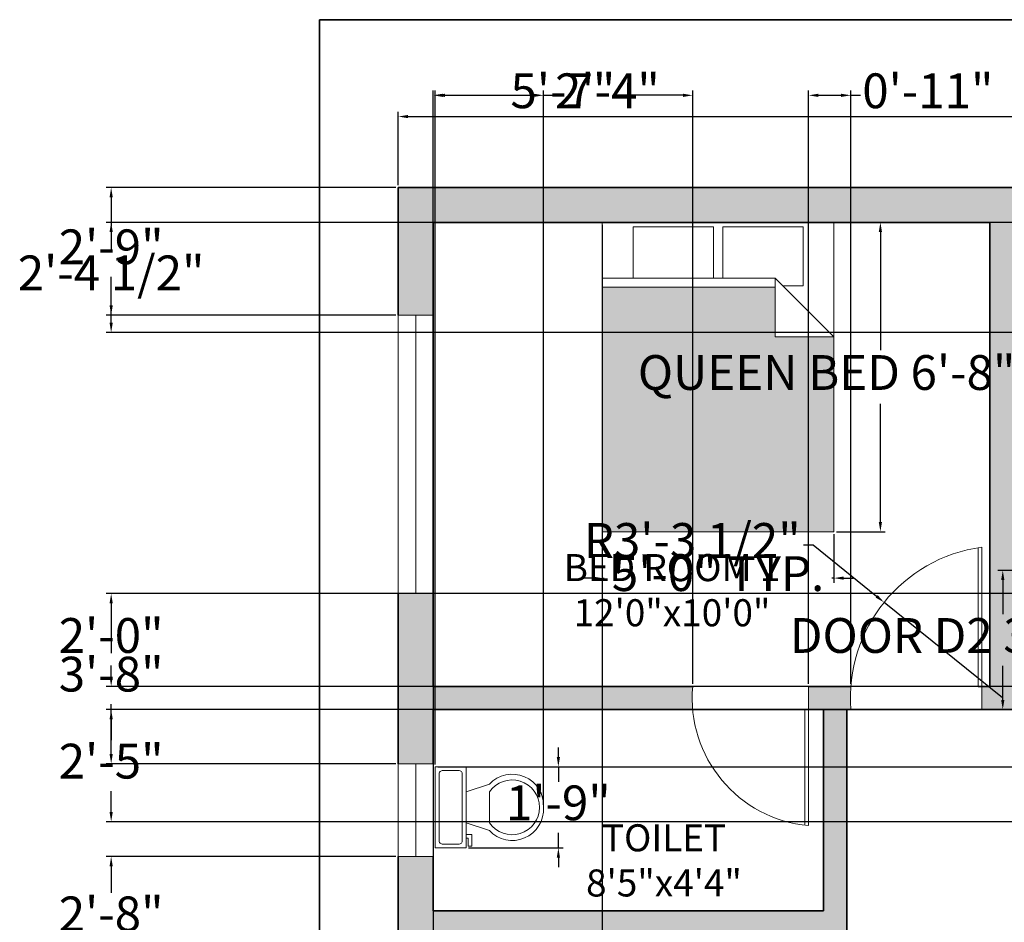
# Model space of a CAD drawing. Units: inches. Extents: x 2151 to 2709, y 3533 to 4046.
# Tile 2 of 4: x 2151 to 2406, y 3812 to 4046. Entities that reach past the tile are written whole.
import ezdxf

# ---------------------------------------------------------------- set-up
doc = ezdxf.new("R2010")
doc.units = ezdxf.units.IN
for name, color, linetype, lineweight in [('A-ANNO-DIMS', 2, 'Continuous', 18), ('A-ANNO-TTLB', 7, 'Continuous', 35), ('A-AREA-IDEN', 7, 'Continuous', 25), ('A-DOOR', 3, 'Continuous', 18), ('A-FLOR-FIXT', 8, 'Continuous', 18), ('A-FURN', 8, 'Continuous', 18), ('A-GLAZ', 4, 'Continuous', 18), ('A-WALL', 7, 'Continuous', 35)]:
    doc.layers.add(name, color=color, linetype=linetype, lineweight=lineweight)
doc.layers.add('A-FURN-PATT', color=107, linetype='Continuous', lineweight=13, true_color=0x477749)
doc.layers.add('A-WALL-PATT', color=18, linetype='Continuous', lineweight=13, true_color=0x000000)
doc.styles.get("Standard").update_dxf_attribs({"font": 'arial.ttf'})
doc.dimstyles.new('ISO-25', dxfattribs={"dimtxt": 9, "dimasz": 2.5, "dimexe": 1.25, "dimexo": 0.625, "dimgap": 2, "dimtad": 0, "dimtih": 1, "dimtoh": 1, "dimdec": 1, "dimlunit": 4, "dimtxsty": 'Standard', "dimcen": 2.5, "dimadec": 0, "dimazin": 0, "dimtfac": 0.5, "dimtdec": 1, "dimtmove": 0, "dimatfit": 3, "dimfxl": 1, "dimarcsym": 0})

# ---------------------------------------------------------------- blocks, each defined once
blk = doc.blocks.new('Bed - Queen')
for p, q in [((0, -80.00003), (0, 0)), ((0, 0), (59.99999, 0)), ((59.99999, 0), (59.99999, -80.00003)), ((7.99999, -1.2), (28.79998, -1.2)), ((7.99999, -14.4), (7.99999, -1.2)), ((28.79998, -1.2), (28.79998, -14.4)), ((31.19999, -1.2), (51.99999, -1.2)), ((31.19999, -14.4), (31.19999, -1.2)), ((51.99999, -1.2), (51.99999, -16.4)), ((0, -14.4), (44.8, -14.4)), ((59.99999, -29.6), (44.8, -14.4)), ((44.8, -14.4), (44.8, -29.6)), ((44.8, -16.8), (0, -16.8)), ((51.99999, -16.4), (46.79936, -16.4)), ((44.8, -29.6), (59.99999, -29.6)), ((59.99999, -80.00003), (0, -80.00003))]:
    blk.add_line(p, q)
blk = doc.blocks.new('*U3')
for p, q in [((9.5, -6), (9.5, -2)), ((-10, -8.5), (-8, -8.5)), ((-10, -9.5), (-10, -8.5)), ((-7, -9.5), (-10, -9.5)), ((-8, -8.5), (-8, -8)), ((-7, -8), (-7, -9.5)), ((-4, -8), (-6, -14)), ((4, -8), (6, -14)), ((4, -14), (-4, -14))]:
    blk.add_line(p, q)
blk.add_lwpolyline([(10.5, -8), (10.5, 0), (-10.5, 0), (-10.5, -8)], close=True)
for points in [[(-9.5, -2), (-9.5, -6)], [(8.5, -1), (-8.5, -1)], [(-8.5, -7), (8.5, -7)]]:
    blk.add_lwpolyline(points)
for centre, radius, start, end in [((-8.625, -1.875), 0.8839, 81.8699, 188.1301), ((8.625, -1.875), 0.8839, 351.8699, 98.1301), ((-8.625, -6.125), 0.8839, 171.869898, 278.1301), ((8.625, -6.125), 0.8839, 261.8699, 8.1301), ((-0.4772, -19.9188), 8.0953, 133.01722, 273.38), ((0.0374, -19.8731), 7.127, 124.50543, 269.7), ((-0.0373, -19.8731), 7.127, 270.3, 55.4946), ((0.4773, -19.9188), 8.0953, 266.62, 46.9828)]:
    blk.add_arc(centre, radius, start, end)
blk = doc.blocks.new('*D6')
at = {"layer": 'A-ANNO-DIMS', "color": 0, "lineweight": -2, "transparency": 16777216}
for p, q in [((2248.83, 4002.79), (2248.83, 4021.77)), ((2251.33, 4020.52), (2431.2, 4020.52)), ((2630.33, 4020.52), (2450.47, 4020.52)), ((2632.83, 4002.79), (2632.83, 4021.77))]:
    blk.add_line(p, q, dxfattribs=at)
at = {"layer": 'A-ANNO-DIMS', "color": 0, "transparency": 16777216}
for points in [[(2251.33, 4020.94), (2251.33, 4020.11), (2248.83, 4020.52)], [(2630.33, 4020.94), (2630.33, 4020.11), (2632.83, 4020.52)]]:
    blk.add_solid(points, dxfattribs=at)
at = {"layer": 'Defpoints', "color": 0, "transparency": 16777216}
for p in [(2632.83, 4020.52), (2248.83, 4002.17), (2632.83, 4002.17)]:
    blk.add_point(p, dxfattribs=at)
at = {"layer": 'A-ANNO-DIMS', "color": 0, "transparency": 16777216, "insert": (2440.83, 4020.52), "char_height": 9, "attachment_point": 5}
blk.add_mtext("32'", dxfattribs=at)
blk = doc.blocks.new('WIN-72IN')
for p, q in [((9, 72), (0, 72)), ((0, 72), (0, 0)), ((4.5, 0), (4.5, 72)), ((9, 72), (9, 0)), ((9, 0), (0, 0))]:
    blk.add_line(p, q)
blk = doc.blocks.new('WIN-24IN')
for p, q in [((0, 0), (0, 9)), ((0, 9), (24, 9)), ((24, 0), (24, 9)), ((0, 4.5), (24, 4.5)), ((0, 0), (24, 0))]:
    blk.add_line(p, q)
blk = doc.blocks.new('DOOR-SWING-30IN')
for p, q in [((0, 6), (0, 36)), ((1, 6), (1, 35.89)), ((0, 6), (0, 0)), ((0, 0), (30, 0))]:
    blk.add_line(p, q)
blk.add_arc((-3, 3), 33.14, 354.8056, 84.8056)
blk = doc.blocks.new('*D19')
at = {"layer": 'A-ANNO-DIMS', "color": 0, "lineweight": -2, "transparency": 16777216}
for p, q in [((2362.18, 3993.17), (2374.8, 3993.17)), ((2373.55, 3990.67), (2373.55, 3960.09)), ((2373.55, 3915.67), (2373.55, 3946.24)), ((2362.18, 3913.17), (2374.8, 3913.17))]:
    blk.add_line(p, q, dxfattribs=at)
at = {"layer": 'A-ANNO-DIMS', "color": 0, "transparency": 16777216}
for points in [[(2373.14, 3990.67), (2373.97, 3990.67), (2373.55, 3993.17)], [(2373.14, 3915.67), (2373.97, 3915.67), (2373.55, 3913.17)]]:
    blk.add_solid(points, dxfattribs=at)
at = {"layer": 'Defpoints', "color": 0, "transparency": 16777216}
for p in [(2361.55, 3993.17), (2373.55, 3993.17), (2361.55, 3913.17)]:
    blk.add_point(p, dxfattribs=at)
at = {"layer": 'A-ANNO-DIMS', "color": 0, "transparency": 16777216, "insert": (2373.55, 3953.17), "char_height": 9, "attachment_point": 5}
blk.add_mtext('QUEEN BED 6\'-8" TYP.', dxfattribs=at)
blk = doc.blocks.new('*D20')
at = {"layer": 'A-ANNO-DIMS', "color": 0, "lineweight": -2, "transparency": 16777216}
for p, q in [((2301.55, 3912.54), (2301.55, 3899.92)), ((2361.55, 3912.54), (2361.55, 3899.92)), ((2299.05, 3901.17), (2296.55, 3901.17)), ((2301.55, 3901.17), (2302.12, 3901.17)), ((2361.55, 3901.17), (2360.98, 3901.17)), ((2364.05, 3901.17), (2366.55, 3901.17))]:
    blk.add_line(p, q, dxfattribs=at)
at = {"layer": 'A-ANNO-DIMS', "color": 0, "transparency": 16777216}
for points in [[(2299.05, 3901.58), (2299.05, 3900.75), (2301.55, 3901.17)], [(2364.05, 3901.58), (2364.05, 3900.75), (2361.55, 3901.17)]]:
    blk.add_solid(points, dxfattribs=at)
at = {"layer": 'Defpoints', "color": 0, "transparency": 16777216}
for p in [(2301.55, 3913.17), (2361.55, 3913.17), (2361.55, 3901.17)]:
    blk.add_point(p, dxfattribs=at)
at = {"layer": 'A-ANNO-DIMS', "color": 0, "transparency": 16777216, "insert": (2331.55, 3901.17), "char_height": 9, "attachment_point": 5}
blk.add_mtext('5\'-0" TYP.', dxfattribs=at)
blk = doc.blocks.new('*D23')
at = {"layer": 'A-ANNO-DIMS', "color": 0, "lineweight": -2, "transparency": 16777216}
for p, q in [((2409.99, 3903.17), (2403.96, 3903.17)), ((2405.21, 3900.67), (2405.21, 3891.82)), ((2405.21, 3869.67), (2405.21, 3878.51)), ((2409.99, 3867.17), (2403.96, 3867.17))]:
    blk.add_line(p, q, dxfattribs=at)
at = {"layer": 'A-ANNO-DIMS', "color": 0, "transparency": 16777216}
for points in [[(2404.79, 3900.67), (2405.63, 3900.67), (2405.21, 3903.17)], [(2404.79, 3869.67), (2405.63, 3869.67), (2405.21, 3867.17)]]:
    blk.add_solid(points, dxfattribs=at)
at = {"layer": 'Defpoints', "color": 0, "transparency": 16777216}
for p in [(2405.21, 3903.17), (2410.61, 3903.17), (2410.61, 3867.17)]:
    blk.add_point(p, dxfattribs=at)
at = {"layer": 'A-ANNO-DIMS', "color": 0, "transparency": 16777216, "insert": (2405.21, 3885.17), "char_height": 9, "attachment_point": 5}
blk.add_mtext('DOOR D2 3\'-0" TYP.', dxfattribs=at)
blk = doc.blocks.new('*D29')
at = {"layer": 'A-ANNO-DIMS', "color": 0, "lineweight": -2, "transparency": 16777216}
for p, q in [((2248.21, 4002.17), (2173.29, 4002.17)), ((2174.54, 3999.67), (2174.54, 3992.26)), ((2174.54, 3971.67), (2174.54, 3979.07)), ((2248.21, 3969.17), (2173.29, 3969.17))]:
    blk.add_line(p, q, dxfattribs=at)
at = {"layer": 'A-ANNO-DIMS', "color": 0, "transparency": 16777216}
for points in [[(2174.13, 3999.67), (2174.96, 3999.67), (2174.54, 4002.17)], [(2174.13, 3971.67), (2174.96, 3971.67), (2174.54, 3969.17)]]:
    blk.add_solid(points, dxfattribs=at)
at = {"layer": 'Defpoints', "color": 0, "transparency": 16777216}
for p in [(2248.83, 4002.17), (2174.54, 3969.17), (2248.83, 3969.17)]:
    blk.add_point(p, dxfattribs=at)
at = {"layer": 'A-ANNO-DIMS', "color": 0, "transparency": 16777216, "insert": (2174.54, 3985.67), "char_height": 9, "attachment_point": 5}
blk.add_mtext('2\'-9"', dxfattribs=at)
blk = doc.blocks.new('*D30')
at = {"layer": 'A-ANNO-DIMS', "color": 0, "lineweight": -2, "transparency": 16777216}
for p, q in [((2623.21, 3867.17), (2173.29, 3867.17)), ((2174.54, 3864.67), (2174.54, 3859.26)), ((2174.54, 3840.67), (2174.54, 3846.07)), ((2623.21, 3838.17), (2173.29, 3838.17))]:
    blk.add_line(p, q, dxfattribs=at)
at = {"layer": 'A-ANNO-DIMS', "color": 0, "transparency": 16777216}
for points in [[(2174.13, 3864.67), (2174.96, 3864.67), (2174.54, 3867.17)], [(2174.13, 3840.67), (2174.96, 3840.67), (2174.54, 3838.17)]]:
    blk.add_solid(points, dxfattribs=at)
at = {"layer": 'Defpoints', "color": 0, "transparency": 16777216}
for p in [(2174.54, 3867.17), (2623.83, 3867.17), (2623.83, 3838.17)]:
    blk.add_point(p, dxfattribs=at)
at = {"layer": 'A-ANNO-DIMS', "color": 0, "transparency": 16777216, "insert": (2174.54, 3852.67), "char_height": 9, "attachment_point": 5}
blk.add_mtext('2\'-5"', dxfattribs=at)
blk = doc.blocks.new('*D31')
at = {"layer": 'A-ANNO-DIMS', "color": 0, "lineweight": -2, "transparency": 16777216}
for p, q in [((2623.21, 3897.17), (2173.29, 3897.17)), ((2174.54, 3894.67), (2174.54, 3891.76)), ((2174.54, 3875.67), (2174.54, 3878.57)), ((2623.21, 3873.17), (2173.29, 3873.17))]:
    blk.add_line(p, q, dxfattribs=at)
at = {"layer": 'A-ANNO-DIMS', "color": 0, "transparency": 16777216}
for points in [[(2174.13, 3894.67), (2174.96, 3894.67), (2174.54, 3897.17)], [(2174.13, 3875.67), (2174.96, 3875.67), (2174.54, 3873.17)]]:
    blk.add_solid(points, dxfattribs=at)
at = {"layer": 'Defpoints', "color": 0, "transparency": 16777216}
for p in [(2174.54, 3897.17), (2623.83, 3897.17), (2623.83, 3873.17)]:
    blk.add_point(p, dxfattribs=at)
at = {"layer": 'A-ANNO-DIMS', "color": 0, "transparency": 16777216, "insert": (2174.54, 3885.17), "char_height": 9, "attachment_point": 5}
blk.add_mtext('2\'-0"', dxfattribs=at)
blk = doc.blocks.new('*D36')
at = {"layer": 'A-ANNO-DIMS', "color": 0, "lineweight": -2, "transparency": 16777216}
for p, q in [((2248.21, 3829.17), (2173.29, 3829.17)), ((2174.54, 3826.67), (2174.54, 3819.76)), ((2174.54, 3799.67), (2174.54, 3806.57)), ((2248.21, 3797.17), (2173.29, 3797.17))]:
    blk.add_line(p, q, dxfattribs=at)
at = {"layer": 'A-ANNO-DIMS', "color": 0, "transparency": 16777216}
for points in [[(2174.13, 3826.67), (2174.96, 3826.67), (2174.54, 3829.17)], [(2174.13, 3799.67), (2174.96, 3799.67), (2174.54, 3797.17)]]:
    blk.add_solid(points, dxfattribs=at)
at = {"layer": 'Defpoints', "color": 0, "transparency": 16777216}
for p in [(2174.54, 3829.17), (2248.83, 3829.17), (2248.83, 3797.17)]:
    blk.add_point(p, dxfattribs=at)
at = {"layer": 'A-ANNO-DIMS', "color": 0, "transparency": 16777216, "insert": (2174.54, 3813.17), "char_height": 9, "attachment_point": 5}
blk.add_mtext('2\'-8"', dxfattribs=at)
blk = doc.blocks.new('*D38')
at = {"layer": 'A-ANNO-DIMS', "color": 0, "lineweight": -2, "transparency": 16777216}
for p, q in [((2248.21, 3897.17), (2173.29, 3897.17)), ((2174.54, 3894.67), (2174.54, 3881.76)), ((2174.54, 3855.67), (2174.54, 3868.57)), ((2248.21, 3853.17), (2173.29, 3853.17))]:
    blk.add_line(p, q, dxfattribs=at)
at = {"layer": 'A-ANNO-DIMS', "color": 0, "transparency": 16777216}
for points in [[(2174.13, 3894.67), (2174.96, 3894.67), (2174.54, 3897.17)], [(2174.13, 3855.67), (2174.96, 3855.67), (2174.54, 3853.17)]]:
    blk.add_solid(points, dxfattribs=at)
at = {"layer": 'Defpoints', "color": 0, "transparency": 16777216}
for p in [(2174.54, 3897.17), (2248.83, 3897.17), (2248.83, 3853.17)]:
    blk.add_point(p, dxfattribs=at)
at = {"layer": 'A-ANNO-DIMS', "color": 0, "transparency": 16777216, "insert": (2174.54, 3875.17), "char_height": 9, "attachment_point": 5}
blk.add_mtext('3\'-8"', dxfattribs=at)
blk = doc.blocks.new('*D40')
at = {"layer": 'A-ANNO-DIMS', "color": 0, "lineweight": -2, "transparency": 16777216}
for p, q in [((2257.83, 3873.79), (2257.83, 4027.27)), ((2260.33, 4026.02), (2277.45, 4026.02)), ((2322.49, 4026.02), (2305.37, 4026.02)), ((2324.99, 3873.79), (2324.99, 4027.27))]:
    blk.add_line(p, q, dxfattribs=at)
at = {"layer": 'A-ANNO-DIMS', "color": 0, "transparency": 16777216}
for points in [[(2260.33, 4026.43), (2260.33, 4025.6), (2257.83, 4026.02)], [(2322.49, 4026.43), (2322.49, 4025.6), (2324.99, 4026.02)]]:
    blk.add_solid(points, dxfattribs=at)
at = {"layer": 'Defpoints', "color": 0, "transparency": 16777216}
for p in [(2324.99, 4026.02), (2257.83, 3873.17), (2324.99, 3873.17)]:
    blk.add_point(p, dxfattribs=at)
at = {"layer": 'A-ANNO-DIMS', "color": 0, "transparency": 16777216, "insert": (2291.41, 4026.02), "char_height": 9, "attachment_point": 5}
blk.add_mtext('5\'-7"', dxfattribs=at)
blk = doc.blocks.new('*D41')
at = {"layer": 'A-ANNO-DIMS', "color": 0, "lineweight": -2, "transparency": 16777216}
for p, q in [((2257.83, 3992.54), (2257.83, 3545.07)), ((2301.55, 3992.54), (2301.55, 3545.07)), ((2260.33, 3546.32), (2299.05, 3546.32)), ((2301.55, 3546.32), (2304.05, 3546.32))]:
    blk.add_line(p, q, dxfattribs=at)
at = {"layer": 'A-ANNO-DIMS', "color": 0, "transparency": 16777216}
for points in [[(2260.33, 3546.73), (2260.33, 3545.9), (2257.83, 3546.32)], [(2299.05, 3546.73), (2299.05, 3545.9), (2301.55, 3546.32)]]:
    blk.add_solid(points, dxfattribs=at)
at = {"layer": 'Defpoints', "color": 0, "transparency": 16777216}
for p in [(2257.83, 3993.17), (2301.55, 3993.17), (2301.55, 3546.32)]:
    blk.add_point(p, dxfattribs=at)
at = {"layer": 'A-ANNO-DIMS', "color": 0, "transparency": 16777216, "insert": (2328.5, 3546.32), "char_height": 9, "attachment_point": 5}
blk.add_mtext('3\'-7 1/2"', dxfattribs=at)
blk = doc.blocks.new('*D44')
at = {"layer": 'A-ANNO-DIMS', "color": 0, "lineweight": -2, "transparency": 16777216}
for p, q in [((2258.39, 3853.01), (2258.39, 4027.27)), ((2260.89, 4026.02), (2283.89, 4026.02)), ((2286.39, 3842.51), (2286.39, 4027.27)), ((2286.39, 4026.02), (2288.89, 4026.02))]:
    blk.add_line(p, q, dxfattribs=at)
at = {"layer": 'A-ANNO-DIMS', "color": 0, "transparency": 16777216}
for points in [[(2260.89, 4026.43), (2260.89, 4025.6), (2258.39, 4026.02)], [(2283.89, 4026.43), (2283.89, 4025.6), (2286.39, 4026.02)]]:
    blk.add_solid(points, dxfattribs=at)
at = {"layer": 'Defpoints', "color": 0, "transparency": 16777216}
for p in [(2286.39, 4026.02), (2258.39, 3852.39), (2286.39, 3841.89)]:
    blk.add_point(p, dxfattribs=at)
at = {"layer": 'A-ANNO-DIMS', "color": 0, "transparency": 16777216, "insert": (2302.93, 4026.02), "char_height": 9, "attachment_point": 5}
blk.add_mtext('2\'-4"', dxfattribs=at)
blk = doc.blocks.new('*D45')
at = {"layer": 'A-ANNO-DIMS', "color": 0, "lineweight": -2, "transparency": 16777216}
for p, q in [((2290.24, 3854.89), (2290.24, 3857.39)), ((2267.02, 3852.39), (2291.49, 3852.39)), ((2290.24, 3852.39), (2290.24, 3848.48)), ((2290.24, 3831.39), (2290.24, 3835.29)), ((2267.02, 3831.39), (2291.49, 3831.39)), ((2290.24, 3828.89), (2290.24, 3826.39))]:
    blk.add_line(p, q, dxfattribs=at)
at = {"layer": 'A-ANNO-DIMS', "color": 0, "transparency": 16777216}
for points in [[(2289.83, 3854.89), (2290.66, 3854.89), (2290.24, 3852.39)], [(2289.83, 3828.89), (2290.66, 3828.89), (2290.24, 3831.39)]]:
    blk.add_solid(points, dxfattribs=at)
at = {"layer": 'Defpoints', "color": 0, "transparency": 16777216}
for p in [(2266.39, 3852.39), (2266.39, 3831.39), (2290.24, 3831.39)]:
    blk.add_point(p, dxfattribs=at)
at = {"layer": 'A-ANNO-DIMS', "color": 0, "transparency": 16777216, "insert": (2290.24, 3841.89), "char_height": 9, "attachment_point": 5}
blk.add_mtext('1\'-9"', dxfattribs=at)
blk = doc.blocks.new('*D48')
at = {"layer": 'A-ANNO-DIMS', "color": 0, "lineweight": -2, "transparency": 16777216}
for p, q in [((2354.99, 3873.79), (2354.99, 4027.27)), ((2357.49, 4026.02), (2363.38, 4026.02)), ((2365.88, 3873.79), (2365.88, 4027.27)), ((2365.88, 4026.02), (2368.38, 4026.02))]:
    blk.add_line(p, q, dxfattribs=at)
at = {"layer": 'A-ANNO-DIMS', "color": 0, "transparency": 16777216}
for points in [[(2357.49, 4026.43), (2357.49, 4025.6), (2354.99, 4026.02)], [(2363.38, 4026.43), (2363.38, 4025.6), (2365.88, 4026.02)]]:
    blk.add_solid(points, dxfattribs=at)
at = {"layer": 'Defpoints', "color": 0, "transparency": 16777216}
for p in [(2365.88, 4026.02), (2354.99, 3873.17), (2365.88, 3873.17)]:
    blk.add_point(p, dxfattribs=at)
at = {"layer": 'A-ANNO-DIMS', "color": 0, "transparency": 16777216, "insert": (2385.84, 4026.02), "char_height": 9, "attachment_point": 5}
blk.add_mtext('0\'-11"', dxfattribs=at)
blk = doc.blocks.new('*D52')
at = {"layer": 'A-ANNO-DIMS', "color": 0, "lineweight": -2, "transparency": 16777216}
for p, q in [((2473.21, 3993.17), (2173.29, 3993.17)), ((2174.54, 3990.67), (2174.54, 3985.58)), ((2174.54, 3967.19), (2174.54, 3972.27)), ((2472.97, 3964.69), (2173.29, 3964.69))]:
    blk.add_line(p, q, dxfattribs=at)
at = {"layer": 'A-ANNO-DIMS', "color": 0, "transparency": 16777216}
for points in [[(2174.13, 3990.67), (2174.96, 3990.67), (2174.54, 3993.17)], [(2174.13, 3967.19), (2174.96, 3967.19), (2174.54, 3964.69)]]:
    blk.add_solid(points, dxfattribs=at)
at = {"layer": 'Defpoints', "color": 0, "transparency": 16777216}
for p in [(2473.83, 3993.17), (2174.54, 3964.69), (2473.59, 3964.69)]:
    blk.add_point(p, dxfattribs=at)
at = {"layer": 'A-ANNO-DIMS', "color": 0, "transparency": 16777216, "insert": (2174.54, 3978.93), "char_height": 9, "attachment_point": 5}
blk.add_mtext('2\'-4 1/2"', dxfattribs=at)
blk = doc.blocks.new('*D53')
at = {"layer": 'A-ANNO-DIMS', "color": 0, "lineweight": -2, "transparency": 16777216}
for p, q in [((2656.68, 3869.67), (2656.68, 3872.17)), ((2258.46, 3867.17), (2657.93, 3867.17)), ((2656.68, 3867.17), (2656.68, 3866.37)), ((2259.02, 3852.39), (2657.93, 3852.39)), ((2656.68, 3852.39), (2656.68, 3853.18)), ((2656.68, 3849.89), (2656.68, 3847.39))]:
    blk.add_line(p, q, dxfattribs=at)
at = {"layer": 'A-ANNO-DIMS', "color": 0, "transparency": 16777216}
for points in [[(2656.26, 3869.67), (2657.1, 3869.67), (2656.68, 3867.17)], [(2656.26, 3849.89), (2657.1, 3849.89), (2656.68, 3852.39)]]:
    blk.add_solid(points, dxfattribs=at)
at = {"layer": 'Defpoints', "color": 0, "transparency": 16777216}
for p in [(2257.83, 3867.17), (2656.68, 3867.17), (2258.39, 3852.39)]:
    blk.add_point(p, dxfattribs=at)
at = {"layer": 'A-ANNO-DIMS', "color": 0, "transparency": 16777216, "insert": (2656.68, 3859.78), "char_height": 9, "attachment_point": 5}
blk.add_mtext('1\'-3"', dxfattribs=at)
blk = doc.blocks.new('*D56')
at = {"layer": 'A-ANNO-DIMS', "color": 0, "lineweight": -2, "transparency": 16777216}
for p, q in [((2353.64, 3909.74), (2356.14, 3909.74)), ((2356.14, 3909.74), (2372.57, 3896.47)), ((2405.13, 3870.17), (2374.51, 3894.9))]:
    blk.add_line(p, q, dxfattribs=at)
at = {"layer": 'A-ANNO-DIMS', "color": 0, "transparency": 16777216}
blk.add_solid([(2372.83, 3896.79), (2372.3, 3896.14), (2374.51, 3894.9)], dxfattribs=at)
at = {"layer": 'Defpoints', "color": 0, "transparency": 16777216}
for p in [(2374.51, 3894.9), (2405.13, 3870.17)]:
    blk.add_point(p, dxfattribs=at)
at = {"layer": 'A-ANNO-DIMS', "color": 0, "transparency": 16777216, "insert": (2324.88, 3909.74), "char_height": 9, "attachment_point": 5}
blk.add_mtext('R3\'-3 1/2"', dxfattribs=at)

msp = doc.modelspace()

# ---------------------------------------------------------------- hatches: boundary and pattern name
at = {"layer": 'A-FURN-PATT'}
h = msp.add_hatch(color=256, dxfattribs=at)
h.dxf.hatch_style = 1
h.paths.add_polyline_path([(2361.55, 3963.57), (2346.35, 3963.57), (2346.35, 3976.37), (2301.55, 3976.37), (2301.55, 3913.17), (2361.55, 3913.17)])
h.paths.add_polyline_path([(2582.34, 3963.57), (2567.14, 3963.57), (2567.14, 3976.37), (2522.34, 3976.37), (2522.34, 3913.17), (2582.34, 3913.17)])
at = {"layer": 'A-WALL-PATT'}
h = msp.add_hatch(color=256, dxfattribs=at)
h.dxf.hatch_style = 1
h.paths.add_polyline_path([(2428.83, 4002.17), (2248.83, 4002.17), (2248.83, 3969.17), (2257.83, 3969.17), (2257.83, 3993.17), (2401.83, 3993.17), (2401.83, 3873.17), (2399.81, 3873.17), (2399.81, 3867.17), (2410.61, 3867.17), (2410.61, 3873.17), (2407.83, 3873.17), (2407.83, 3993.17), (2428.83, 3993.17)])
h.paths.add_polyline_path([(2632.83, 4002.17), (2452.83, 4002.17), (2452.83, 3993.17), (2473.83, 3993.17), (2473.83, 3873.17), (2440.61, 3873.17, -0.045361), (2440.61, 3867.17), (2482.29, 3867.17), (2482.29, 3873.17), (2479.83, 3873.17), (2479.83, 3993.17), (2623.83, 3993.17), (2623.83, 3969.17), (2632.83, 3969.17)])
h.paths.add_polyline_path([(2257.83, 3897.17), (2248.83, 3897.17), (2248.83, 3853.17), (2257.83, 3853.17), (2257.83, 3867.17), (2324.99, 3867.17, -0.045361), (2324.99, 3873.17), (2257.83, 3873.17)])
h.paths.add_polyline_path([(2632.83, 3897.17), (2623.83, 3897.17), (2623.83, 3873.17), (2518.29, 3873.17, -0.038405), (2518.29, 3867.17), (2623.83, 3867.17), (2623.83, 3838.17), (2632.83, 3838.17)])
h.paths.add_polyline_path([(2364.83, 3815.17), (2364.83, 3867.17), (2365.88, 3867.17, -0.038164), (2365.88, 3873.17), (2354.99, 3873.17), (2354.99, 3867.17), (2358.83, 3867.17), (2358.83, 3815.17), (2257.83, 3815.17), (2257.83, 3829.17), (2248.83, 3829.17), (2248.83, 3797.17), (2257.83, 3797.17), (2257.83, 3809.17), (2358.83, 3809.17), (2364.83, 3809.17)])
h.paths.add_polyline_path([(2364.21, 3737.17), (2257.83, 3737.17), (2257.83, 3749.17), (2248.83, 3749.17), (2248.83, 3685.17), (2257.83, 3685.17), (2257.83, 3731.17), (2364.21, 3731.17, -0.038405)])
h.paths.add_polyline_path([(2257.83, 3625.17), (2248.83, 3625.17), (2248.83, 3570.17), (2299.83, 3570.17), (2299.83, 3579.17), (2257.83, 3579.17)])

# ---------------------------------------------------------------- linework, layer by layer
at = {"layer": 'A-ANNO-TTLB'}
msp.add_lwpolyline([(2228.43, 4045.57), (2671.96, 4045.57), (2671.96, 3550.81), (2228.43, 3550.81)], close=True, dxfattribs=at)
at = {"layer": 'A-DOOR'}
for p, q in [((2398.81, 3873.17), (2398.81, 3909.02)), ((2399.81, 3873.17), (2399.81, 3909.17)), ((2399.81, 3873.17), (2399.81, 3867.17)), ((2365.88, 3867.17), (2399.81, 3867.17))]:
    msp.add_line(p, q, dxfattribs=at)
msp.add_arc((2405.13, 3870.17), 39.36, 97.7723, 184.3711, dxfattribs=at)
at = {"layer": 'A-WALL'}
for p, q in [((2248.83, 4002.17), (2428.83, 4002.17)), ((2248.83, 3969.17), (2248.83, 4002.17)), ((2257.83, 3993.17), (2401.83, 3993.17)), ((2257.83, 3993.17), (2401.83, 3993.17)), ((2257.83, 3969.17), (2257.83, 3993.17)), ((2401.83, 3873.17), (2401.83, 3993.17)), ((2248.83, 3853.17), (2248.83, 3897.17)), ((2257.83, 3873.17), (2257.83, 3897.17)), ((2257.83, 3873.17), (2324.99, 3873.17)), ((2354.99, 3873.17), (2365.88, 3873.17)), ((2398.81, 3873.17), (2401.83, 3873.17)), ((2257.83, 3867.17), (2324.99, 3867.17)), ((2257.83, 3853.17), (2257.83, 3867.17)), ((2353.99, 3867.17), (2358.83, 3867.17)), ((2358.83, 3815.17), (2358.83, 3867.17)), ((2364.83, 3815.17), (2364.83, 3867.17)), ((2364.83, 3867.17), (2365.88, 3867.17)), ((2399.81, 3867.17), (2410.61, 3867.17)), ((2248.83, 3797.17), (2248.83, 3829.17)), ((2257.83, 3815.17), (2257.83, 3829.17)), ((2257.83, 3815.17), (2358.83, 3815.17)), ((2364.83, 3815.17), (2364.83, 3809.17))]:
    msp.add_line(p, q, dxfattribs=at)

# ---------------------------------------------------------------- block references
at = {"layer": 'A-DOOR', "rotation": 180}
msp.add_blockref('DOOR-SWING-30IN', (2354.99, 3873.17), dxfattribs=at)
at = {"layer": 'A-FLOR-FIXT', "rotation": 89.99999999999999}
msp.add_blockref('*U3', (2258.39, 3841.89), dxfattribs=at)
at = {"layer": 'A-FURN'}
msp.add_blockref('Bed - Queen', (2301.55, 3993.17), dxfattribs=at)
at = {"layer": 'A-GLAZ'}
msp.add_blockref('WIN-72IN', (2248.83, 3897.17), dxfattribs=at)
at = {"layer": 'A-GLAZ', "rotation": 90.00000000000072}
msp.add_blockref('WIN-24IN', (2257.83, 3829.17), dxfattribs=at)

# ---------------------------------------------------------------- texts
at = {"layer": 'A-AREA-IDEN', "char_height": 7, "attachment_point": 1}
for s, width, insert in [('\\pxqc;{\\fArial|b1|i0|c0|p34;BED ROOM 1\\P12\'0"x10\'0"}', 79.1963, (2280.05, 3907.38)), ('\\pxqc;{\\fArial|b1|i0|c0|p34;TOILET\\P8\'5"x4\'4"}', 53.1566, (2290.99, 3837.51))]:
    msp.add_mtext_dynamic_manual_height_columns(s, width=width, gutter_width=12.5, heights=[0], dxfattribs=dict(at, insert=insert))

# ---------------------------------------------------------------- dimensions: what is measured, and where the dimension line sits
at = {"layer": 'A-ANNO-DIMS'}
for base, p1, p2, override, picture, middle in [((2324.99, 4026.02), (2257.83, 3873.17), (2324.99, 3873.17), {"dimdec": 1, "dimlfac": 1, "dimrnd": 0, "dimzin": 1, "dimdsep": 46, "dimlunit": 4, "dimfrac": 2}, '*D40', (2291.41, 4026.02)), ((2286.39, 4026.02), (2258.39, 3852.39), (2286.39, 3841.89), {"dimdec": 1, "dimlfac": 1, "dimrnd": 0, "dimzin": 1, "dimdsep": 46, "dimlunit": 4, "dimfrac": 2}, '*D44', (2302.93, 4026.02)), ((2365.88, 4026.02), (2354.99, 3873.17), (2365.88, 3873.17), {"dimdec": 1, "dimlfac": 1, "dimrnd": 0, "dimzin": 1, "dimdsep": 46, "dimlunit": 4, "dimfrac": 2}, '*D48', (2385.84, 4026.02)), ((2632.83, 4020.52), (2248.83, 4002.17), (2632.83, 4002.17), {"dimclrd": 0, "dimclre": 0, "dimclrt": 0}, '*D6', (2440.83, 4020.52)), ((2301.55, 3546.32), (2257.83, 3993.17), (2301.55, 3993.17), {"dimdec": 1, "dimlfac": 1, "dimrnd": 0, "dimzin": 1, "dimdsep": 46, "dimlunit": 4, "dimfrac": 2}, '*D41', (2328.5, 3546.32))]:
    dim = msp.add_linear_dim(base=base, p1=p1, p2=p2, dimstyle='ISO-25', override=override, dxfattribs=at)
    dim.commit()
    dim.dimension.update_dxf_attribs({"geometry": picture, "text_midpoint": middle})
for base, p1, p2, angle, picture, middle in [((2174.54, 3969.17), (2248.83, 4002.17), (2248.83, 3969.17), 90, '*D29', (2174.54, 3985.67)), ((2174.54, 3964.69), (2473.83, 3993.17), (2473.59, 3964.69), 90, '*D52', (2174.54, 3978.93)), ((2174.54, 3897.17), (2623.83, 3873.17), (2623.83, 3897.17), 90, '*D31', (2174.54, 3885.17)), ((2174.54, 3897.17), (2248.83, 3853.17), (2248.83, 3897.17), 90, '*D38', (2174.54, 3875.17)), ((2656.68, 3867.17), (2258.39, 3852.39), (2257.83, 3867.17), 90, '*D53', (2656.68, 3859.78)), ((2174.54, 3867.17), (2623.83, 3838.17), (2623.83, 3867.17), 90, '*D30', (2174.54, 3852.67)), ((2290.24, 3831.39), (2266.39, 3852.39), (2266.39, 3831.39), 270, '*D45', (2290.24, 3841.89)), ((2174.54, 3829.17), (2248.83, 3797.17), (2248.83, 3829.17), 90, '*D36', (2174.54, 3813.17))]:
    dim = msp.add_linear_dim(base=base, p1=p1, p2=p2, angle=angle, dimstyle='ISO-25', override={"dimdec": 1, "dimlfac": 1, "dimrnd": 0, "dimzin": 1, "dimdsep": 46, "dimlunit": 4, "dimfrac": 2}, dxfattribs=at)
    dim.commit()
    dim.dimension.update_dxf_attribs({"geometry": picture, "text_midpoint": middle})
for base, p1, p2, text, picture, middle in [((2373.55, 3993.17), (2361.55, 3913.17), (2361.55, 3993.17), 'QUEEN BED <> TYP.', '*D19', (2373.55, 3953.17)), ((2405.21, 3903.17), (2410.61, 3867.17), (2410.61, 3903.17), 'DOOR D2 <> TYP.', '*D23', (2405.21, 3885.17))]:
    dim = msp.add_linear_dim(base=base, p1=p1, p2=p2, angle=90, text=text, dimstyle='ISO-25', override={"dimdec": 1, "dimlfac": 1, "dimrnd": 0, "dimzin": 1, "dimdsep": 46, "dimlunit": 4, "dimfrac": 2}, dxfattribs=at)
    dim.commit()
    dim.dimension.update_dxf_attribs({"geometry": picture, "text_midpoint": middle})
dim = msp.add_radius_dim(center=(2405.13, 3870.17), mpoint=(2374.51, 3894.9), dimstyle='ISO-25', override={"dimdec": 1, "dimlfac": 1, "dimrnd": 0, "dimzin": 1, "dimdsep": 46, "dimlunit": 4, "dimfrac": 2}, dxfattribs=at)
dim.commit()
dim.dimension.update_dxf_attribs({"geometry": '*D56', "text_midpoint": (2324.88, 3909.74), "dimtype": 164})
dim = msp.add_linear_dim(base=(2361.55, 3901.17), p1=(2301.55, 3913.17), p2=(2361.55, 3913.17), text='<> TYP.', dimstyle='ISO-25', override={"dimdec": 1, "dimlfac": 1, "dimrnd": 0, "dimzin": 1, "dimdsep": 46, "dimlunit": 4, "dimfrac": 2}, dxfattribs=at)
dim.commit()
dim.dimension.update_dxf_attribs({"geometry": '*D20', "text_midpoint": (2331.55, 3901.17)})

doc.saveas('drawing.dxf')
